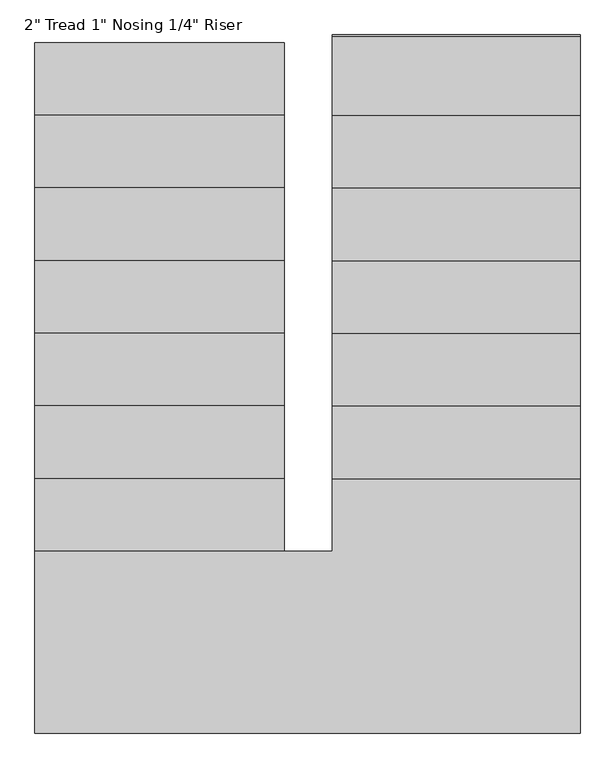
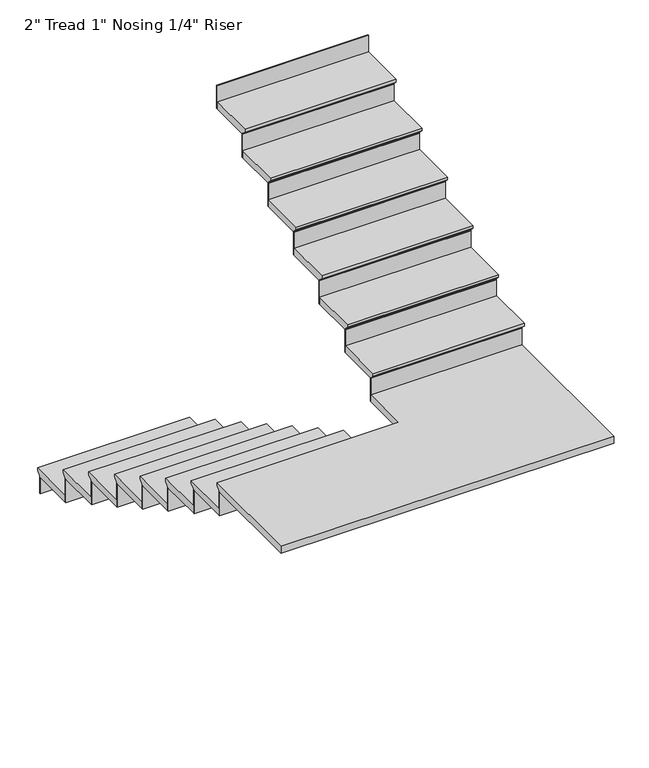
"""IFC4 building model written with IfcOpenShell, lengths in millimetres: stair flight geometry."""

from ifc_helpers import new_model, si_unit, origin, place, context, project, spatial, faceted_brep, source, transform, mapped, element, save


def stair_flight_c3010b6b(model_context):
    return source(origin(), model_context, "Body", "Brep", [
        faceted_brep([(-4232.280864, -3571.6080018, 6398.6833333), (-4232.280864, -3571.6080018, 6417.7333333), (-3187.6083919, -3571.6080018, 6417.7333333), (-3187.6083919, -3571.6080018, 6398.6833333), (-4232.280864, -3597.0080018, 6373.2833333), (-3187.6083919, -3597.0080018, 6373.2833333), (-4232.280864, -3901.8080018, 6417.7333333), (-3187.6083919, -3901.8080018, 6417.7333333), (-3187.6083919, -3597.0080018, 6366.9333333), (-3187.6083919, -3901.8080018, 6366.9333333), (-4232.280864, -3901.8080018, 6366.9333333), (-4232.280864, -3597.0080018, 6366.9333333)], [[[0, 1, 2, 3]], [[4, 0, 3, 5]], [[2, 1, 6, 7]], [[8, 9, 10, 11]], [[2, 7, 9, 8, 5, 3]], [[8, 11, 4, 5]], [[6, 1, 0, 4, 11, 10]], [[7, 6, 10, 9]]]),
        faceted_brep([(-4232.280864, -3597.0080018, 6366.9333333), (-4232.280864, -3597.0080018, 6248.4), (-4232.280864, -3603.3580018, 6248.4), (-4232.280864, -3603.3580018, 6366.9333333), (-3187.6083919, -3597.0080018, 6366.9333333), (-3187.6083919, -3603.3580018, 6366.9333333), (-3187.6083919, -3603.3580018, 6248.4), (-3187.6083919, -3597.0080018, 6248.4)], [[[0, 1, 2, 3]], [[4, 5, 6, 7]], [[1, 0, 4, 7]], [[2, 1, 7, 6]], [[3, 2, 6, 5]], [[0, 3, 5, 4]]]),
        faceted_brep([(-4232.280864, -3901.8080018, 6536.2666667), (-4232.280864, -3901.8080018, 6366.9333333), (-4232.280864, -3908.1580018, 6366.9333333), (-4232.280864, -3908.1580018, 6536.2666667), (-3187.6083919, -3901.8080018, 6536.2666667), (-3187.6083919, -3908.1580018, 6536.2666667), (-3187.6083919, -3908.1580018, 6366.9333333), (-3187.6083919, -3901.8080018, 6366.9333333)], [[[0, 1, 2, 3]], [[4, 5, 6, 7]], [[1, 0, 4, 7]], [[2, 1, 7, 6]], [[3, 2, 6, 5]], [[0, 3, 5, 4]]]),
        faceted_brep([(-3187.6083919, -3876.4080018, 6587.0666667), (-4232.280864, -3876.4080018, 6587.0666667), (-4232.280864, -4206.6080018, 6587.0666667), (-3187.6083919, -4206.6080018, 6587.0666667), (-3187.6083919, -3901.8080018, 6536.2666667), (-3187.6083919, -4206.6080018, 6536.2666667), (-4232.280864, -4206.6080018, 6536.2666667), (-4232.280864, -3901.8080018, 6536.2666667), (-3187.6083919, -3901.8080018, 6542.6166667), (-3187.6083919, -3876.4080018, 6568.0166667), (-4232.280864, -3901.8080018, 6542.6166667), (-4232.280864, -3876.4080018, 6568.0166667)], [[[0, 1, 2, 3]], [[4, 5, 6, 7]], [[0, 3, 5, 4, 8, 9]], [[4, 7, 10, 8]], [[2, 1, 11, 10, 7, 6]], [[3, 2, 6, 5]], [[11, 1, 0, 9]], [[10, 11, 9, 8]]]),
        faceted_brep([(-4232.280864, -4206.6080018, 6705.6), (-4232.280864, -4206.6080018, 6536.2666667), (-4232.280864, -4212.9580018, 6536.2666667), (-4232.280864, -4212.9580018, 6705.6), (-3187.6083919, -4206.6080018, 6705.6), (-3187.6083919, -4212.9580018, 6705.6), (-3187.6083919, -4212.9580018, 6536.2666667), (-3187.6083919, -4206.6080018, 6536.2666667)], [[[0, 1, 2, 3]], [[4, 5, 6, 7]], [[1, 0, 4, 7]], [[2, 1, 7, 6]], [[3, 2, 6, 5]], [[0, 3, 5, 4]]]),
        faceted_brep([(-3187.6083919, -4181.2080018, 6756.4), (-4232.280864, -4181.2080018, 6756.4), (-4232.280864, -4511.4080018, 6756.4), (-3187.6083919, -4511.4080018, 6756.4), (-3187.6083919, -4206.6080018, 6705.6), (-3187.6083919, -4511.4080018, 6705.6), (-4232.280864, -4511.4080018, 6705.6), (-4232.280864, -4206.6080018, 6705.6), (-3187.6083919, -4206.6080018, 6711.95), (-3187.6083919, -4181.2080018, 6737.35), (-4232.280864, -4206.6080018, 6711.95), (-4232.280864, -4181.2080018, 6737.35)], [[[0, 1, 2, 3]], [[4, 5, 6, 7]], [[0, 3, 5, 4, 8, 9]], [[4, 7, 10, 8]], [[2, 1, 11, 10, 7, 6]], [[3, 2, 6, 5]], [[11, 1, 0, 9]], [[10, 11, 9, 8]]]),
        faceted_brep([(-4232.280864, -4511.4080018, 6874.9333333), (-4232.280864, -4511.4080018, 6705.6), (-4232.280864, -4517.7580018, 6705.6), (-4232.280864, -4517.7580018, 6874.9333333), (-3187.6083919, -4511.4080018, 6874.9333333), (-3187.6083919, -4517.7580018, 6874.9333333), (-3187.6083919, -4517.7580018, 6705.6), (-3187.6083919, -4511.4080018, 6705.6)], [[[0, 1, 2, 3]], [[4, 5, 6, 7]], [[1, 0, 4, 7]], [[2, 1, 7, 6]], [[3, 2, 6, 5]], [[0, 3, 5, 4]]]),
        faceted_brep([(-3187.6083919, -4486.0080018, 6925.7333333), (-4232.280864, -4486.0080018, 6925.7333333), (-4232.280864, -4816.2080018, 6925.7333333), (-3187.6083919, -4816.2080018, 6925.7333333), (-3187.6083919, -4511.4080018, 6874.9333333), (-3187.6083919, -4816.2080018, 6874.9333333), (-4232.280864, -4816.2080018, 6874.9333333), (-4232.280864, -4511.4080018, 6874.9333333), (-3187.6083919, -4511.4080018, 6881.2833333), (-3187.6083919, -4486.0080018, 6906.6833333), (-4232.280864, -4511.4080018, 6881.2833333), (-4232.280864, -4486.0080018, 6906.6833333)], [[[0, 1, 2, 3]], [[4, 5, 6, 7]], [[0, 3, 5, 4, 8, 9]], [[4, 7, 10, 8]], [[2, 1, 11, 10, 7, 6]], [[3, 2, 6, 5]], [[11, 1, 0, 9]], [[10, 11, 9, 8]]]),
        faceted_brep([(-4232.280864, -4816.2080018, 7044.2666667), (-4232.280864, -4816.2080018, 6874.9333333), (-4232.280864, -4822.5580018, 6874.9333333), (-4232.280864, -4822.5580018, 7044.2666667), (-3187.6083919, -4816.2080018, 7044.2666667), (-3187.6083919, -4822.5580018, 7044.2666667), (-3187.6083919, -4822.5580018, 6874.9333333), (-3187.6083919, -4816.2080018, 6874.9333333)], [[[0, 1, 2, 3]], [[4, 5, 6, 7]], [[1, 0, 4, 7]], [[2, 1, 7, 6]], [[3, 2, 6, 5]], [[0, 3, 5, 4]]]),
        faceted_brep([(-3187.6083919, -4790.8080018, 7095.0666667), (-4232.280864, -4790.8080018, 7095.0666667), (-4232.280864, -5121.0080018, 7095.0666667), (-3187.6083919, -5121.0080018, 7095.0666667), (-3187.6083919, -4816.2080018, 7044.2666667), (-3187.6083919, -5121.0080018, 7044.2666667), (-4232.280864, -5121.0080018, 7044.2666667), (-4232.280864, -4816.2080018, 7044.2666667), (-3187.6083919, -4816.2080018, 7050.6166667), (-3187.6083919, -4790.8080018, 7076.0166667), (-4232.280864, -4816.2080018, 7050.6166667), (-4232.280864, -4790.8080018, 7076.0166667)], [[[0, 1, 2, 3]], [[4, 5, 6, 7]], [[0, 3, 5, 4, 8, 9]], [[4, 7, 10, 8]], [[2, 1, 11, 10, 7, 6]], [[3, 2, 6, 5]], [[11, 1, 0, 9]], [[10, 11, 9, 8]]]),
        faceted_brep([(-4232.280864, -5121.0080018, 7213.6), (-4232.280864, -5121.0080018, 7044.2666667), (-4232.280864, -5127.3580018, 7044.2666667), (-4232.280864, -5127.3580018, 7213.6), (-3187.6083919, -5121.0080018, 7213.6), (-3187.6083919, -5127.3580018, 7213.6), (-3187.6083919, -5127.3580018, 7044.2666667), (-3187.6083919, -5121.0080018, 7044.2666667)], [[[0, 1, 2, 3]], [[4, 5, 6, 7]], [[1, 0, 4, 7]], [[2, 1, 7, 6]], [[3, 2, 6, 5]], [[0, 3, 5, 4]]]),
        faceted_brep([(-3187.6083919, -5095.6080018, 7264.4), (-4232.280864, -5095.6080018, 7264.4), (-4232.280864, -5425.8080018, 7264.4), (-3187.6083919, -5425.8080018, 7264.4), (-3187.6083919, -5121.0080018, 7213.6), (-3187.6083919, -5425.8080018, 7213.6), (-4232.280864, -5425.8080018, 7213.6), (-4232.280864, -5121.0080018, 7213.6), (-3187.6083919, -5121.0080018, 7219.95), (-3187.6083919, -5095.6080018, 7245.35), (-4232.280864, -5121.0080018, 7219.95), (-4232.280864, -5095.6080018, 7245.35)], [[[0, 1, 2, 3]], [[4, 5, 6, 7]], [[0, 3, 5, 4, 8, 9]], [[4, 7, 10, 8]], [[2, 1, 11, 10, 7, 6]], [[3, 2, 6, 5]], [[11, 1, 0, 9]], [[10, 11, 9, 8]]]),
        faceted_brep([(-4232.280864, -5425.8080018, 7382.9333333), (-4232.280864, -5425.8080018, 7213.6), (-4232.280864, -5432.1580018, 7213.6), (-4232.280864, -5432.1580018, 7382.9333333), (-3187.6083919, -5425.8080018, 7382.9333333), (-3187.6083919, -5432.1580018, 7382.9333333), (-3187.6083919, -5432.1580018, 7213.6), (-3187.6083919, -5425.8080018, 7213.6)], [[[0, 1, 2, 3]], [[4, 5, 6, 7]], [[1, 0, 4, 7]], [[2, 1, 7, 6]], [[3, 2, 6, 5]], [[0, 3, 5, 4]]]),
        faceted_brep([(-3187.6083919, -5400.4080018, 7433.7333333), (-4232.280864, -5400.4080018, 7433.7333333), (-4232.280864, -5730.6080018, 7433.7333333), (-3187.6083919, -5730.6080018, 7433.7333333), (-3187.6083919, -5425.8080018, 7382.9333333), (-3187.6083919, -5730.6080018, 7382.9333333), (-4232.280864, -5730.6080018, 7382.9333333), (-4232.280864, -5425.8080018, 7382.9333333), (-3187.6083919, -5425.8080018, 7389.2833333), (-3187.6083919, -5400.4080018, 7414.6833333), (-4232.280864, -5425.8080018, 7389.2833333), (-4232.280864, -5400.4080018, 7414.6833333)], [[[0, 1, 2, 3]], [[4, 5, 6, 7]], [[0, 3, 5, 4, 8, 9]], [[4, 7, 10, 8]], [[2, 1, 11, 10, 7, 6]], [[3, 2, 6, 5]], [[11, 1, 0, 9]], [[10, 11, 9, 8]]]),
        faceted_brep([(-4232.280864, -5730.6080018, 7552.2666667), (-4232.280864, -5730.6080018, 7382.9333333), (-4232.280864, -5736.9580018, 7382.9333333), (-4232.280864, -5736.9580018, 7552.2666667), (-3187.6083919, -5730.6080018, 7552.2666667), (-3187.6083919, -5736.9580018, 7552.2666667), (-3187.6083919, -5736.9580018, 7382.9333333), (-3187.6083919, -5730.6080018, 7382.9333333)], [[[0, 1, 2, 3]], [[4, 5, 6, 7]], [[1, 0, 4, 7]], [[2, 1, 7, 6]], [[3, 2, 6, 5]], [[0, 3, 5, 4]]]),
        faceted_brep([(-2984.4083919, -5375.0080018, 7603.0666667), (-2984.4083919, -5705.2080018, 7603.0666667), (-4232.280864, -5705.2080018, 7603.0666667), (-4232.280864, -6467.2080018, 7603.0666667), (-1946.280864, -6467.2080018, 7603.0666667), (-1946.280864, -5375.0080018, 7603.0666667), (-2984.4083919, -5705.2080018, 7552.2666667), (-2984.4083919, -5375.0080018, 7552.2666667), (-1946.280864, -5375.0080018, 7552.2666667), (-1946.280864, -6467.2080018, 7552.2666667), (-4232.280864, -6467.2080018, 7552.2666667), (-4232.280864, -5730.6080018, 7552.2666667), (-3187.6083919, -5730.6080018, 7552.2666667), (-3187.6083919, -5705.2080018, 7552.2666667), (-3187.6083919, -5705.2080018, 7584.0166667), (-4232.280864, -5705.2080018, 7584.0166667), (-3187.6083919, -5730.6080018, 7558.6166667), (-4232.280864, -5730.6080018, 7558.6166667)], [[[0, 1, 2, 3, 4, 5]], [[6, 7, 8, 9, 10, 11, 12, 13]], [[1, 0, 7, 6]], [[2, 1, 6, 13, 14, 15]], [[13, 12, 16, 14]], [[12, 11, 17, 16]], [[3, 2, 15, 17, 11, 10]], [[4, 3, 10, 9]], [[5, 4, 9, 8]], [[0, 5, 8, 7]], [[17, 15, 14, 16]]]),
        faceted_brep([(-1946.280864, -5375.0080018, 7721.6), (-1946.280864, -5375.0080018, 7552.2666667), (-1946.280864, -5368.6580018, 7552.2666667), (-1946.280864, -5368.6580018, 7721.6), (-2984.4083919, -5375.0080018, 7721.6), (-2984.4083919, -5368.6580018, 7721.6), (-2984.4083919, -5368.6580018, 7552.2666667), (-2984.4083919, -5375.0080018, 7552.2666667)], [[[0, 1, 2, 3]], [[4, 5, 6, 7]], [[1, 0, 4, 7]], [[2, 1, 7, 6]], [[3, 2, 6, 5]], [[0, 3, 5, 4]]]),
        faceted_brep([(-2984.4083919, -5400.4080018, 7772.4), (-1946.280864, -5400.4080018, 7772.4), (-1946.280864, -5070.2080018, 7772.4), (-2984.4083919, -5070.2080018, 7772.4), (-2984.4083919, -5375.0080018, 7721.6), (-2984.4083919, -5070.2080018, 7721.6), (-1946.280864, -5070.2080018, 7721.6), (-1946.280864, -5375.0080018, 7721.6), (-2984.4083919, -5375.0080018, 7727.95), (-2984.4083919, -5400.4080018, 7753.35), (-1946.280864, -5375.0080018, 7727.95), (-1946.280864, -5400.4080018, 7753.35)], [[[0, 1, 2, 3]], [[4, 5, 6, 7]], [[0, 3, 5, 4, 8, 9]], [[4, 7, 10, 8]], [[2, 1, 11, 10, 7, 6]], [[3, 2, 6, 5]], [[11, 1, 0, 9]], [[10, 11, 9, 8]]]),
        faceted_brep([(-1946.280864, -5070.2080018, 7890.9333333), (-1946.280864, -5070.2080018, 7721.6), (-1946.280864, -5063.8580018, 7721.6), (-1946.280864, -5063.8580018, 7890.9333333), (-2984.4083919, -5070.2080018, 7890.9333333), (-2984.4083919, -5063.8580018, 7890.9333333), (-2984.4083919, -5063.8580018, 7721.6), (-2984.4083919, -5070.2080018, 7721.6)], [[[0, 1, 2, 3]], [[4, 5, 6, 7]], [[1, 0, 4, 7]], [[2, 1, 7, 6]], [[3, 2, 6, 5]], [[0, 3, 5, 4]]]),
        faceted_brep([(-2984.4083919, -5095.6080018, 7941.7333333), (-1946.280864, -5095.6080018, 7941.7333333), (-1946.280864, -4765.4080018, 7941.7333333), (-2984.4083919, -4765.4080018, 7941.7333333), (-2984.4083919, -5070.2080018, 7890.9333333), (-2984.4083919, -4765.4080018, 7890.9333333), (-1946.280864, -4765.4080018, 7890.9333333), (-1946.280864, -5070.2080018, 7890.9333333), (-2984.4083919, -5070.2080018, 7897.2833333), (-2984.4083919, -5095.6080018, 7922.6833333), (-1946.280864, -5070.2080018, 7897.2833333), (-1946.280864, -5095.6080018, 7922.6833333)], [[[0, 1, 2, 3]], [[4, 5, 6, 7]], [[0, 3, 5, 4, 8, 9]], [[4, 7, 10, 8]], [[2, 1, 11, 10, 7, 6]], [[3, 2, 6, 5]], [[11, 1, 0, 9]], [[10, 11, 9, 8]]]),
        faceted_brep([(-1946.280864, -4765.4080018, 8060.2666667), (-1946.280864, -4765.4080018, 7890.9333333), (-1946.280864, -4759.0580018, 7890.9333333), (-1946.280864, -4759.0580018, 8060.2666667), (-2984.4083919, -4765.4080018, 8060.2666667), (-2984.4083919, -4759.0580018, 8060.2666667), (-2984.4083919, -4759.0580018, 7890.9333333), (-2984.4083919, -4765.4080018, 7890.9333333)], [[[0, 1, 2, 3]], [[4, 5, 6, 7]], [[1, 0, 4, 7]], [[2, 1, 7, 6]], [[3, 2, 6, 5]], [[0, 3, 5, 4]]]),
        faceted_brep([(-2984.4083919, -4790.8080018, 8111.0666667), (-1946.280864, -4790.8080018, 8111.0666667), (-1946.280864, -4460.6080018, 8111.0666667), (-2984.4083919, -4460.6080018, 8111.0666667), (-2984.4083919, -4765.4080018, 8060.2666667), (-2984.4083919, -4460.6080018, 8060.2666667), (-1946.280864, -4460.6080018, 8060.2666667), (-1946.280864, -4765.4080018, 8060.2666667), (-2984.4083919, -4765.4080018, 8066.6166667), (-2984.4083919, -4790.8080018, 8092.0166667), (-1946.280864, -4765.4080018, 8066.6166667), (-1946.280864, -4790.8080018, 8092.0166667)], [[[0, 1, 2, 3]], [[4, 5, 6, 7]], [[0, 3, 5, 4, 8, 9]], [[4, 7, 10, 8]], [[2, 1, 11, 10, 7, 6]], [[3, 2, 6, 5]], [[11, 1, 0, 9]], [[10, 11, 9, 8]]]),
        faceted_brep([(-1946.280864, -4460.6080018, 8229.6), (-1946.280864, -4460.6080018, 8060.2666667), (-1946.280864, -4454.2580018, 8060.2666667), (-1946.280864, -4454.2580018, 8229.6), (-2984.4083919, -4460.6080018, 8229.6), (-2984.4083919, -4454.2580018, 8229.6), (-2984.4083919, -4454.2580018, 8060.2666667), (-2984.4083919, -4460.6080018, 8060.2666667)], [[[0, 1, 2, 3]], [[4, 5, 6, 7]], [[1, 0, 4, 7]], [[2, 1, 7, 6]], [[3, 2, 6, 5]], [[0, 3, 5, 4]]]),
        faceted_brep([(-2984.4083919, -4486.0080018, 8280.4), (-1946.280864, -4486.0080018, 8280.4), (-1946.280864, -4155.8080018, 8280.4), (-2984.4083919, -4155.8080018, 8280.4), (-2984.4083919, -4460.6080018, 8229.6), (-2984.4083919, -4155.8080018, 8229.6), (-1946.280864, -4155.8080018, 8229.6), (-1946.280864, -4460.6080018, 8229.6), (-2984.4083919, -4460.6080018, 8235.95), (-2984.4083919, -4486.0080018, 8261.35), (-1946.280864, -4460.6080018, 8235.95), (-1946.280864, -4486.0080018, 8261.35)], [[[0, 1, 2, 3]], [[4, 5, 6, 7]], [[0, 3, 5, 4, 8, 9]], [[4, 7, 10, 8]], [[2, 1, 11, 10, 7, 6]], [[3, 2, 6, 5]], [[11, 1, 0, 9]], [[10, 11, 9, 8]]]),
        faceted_brep([(-1946.280864, -4155.8080018, 8398.9333333), (-1946.280864, -4155.8080018, 8229.6), (-1946.280864, -4149.4580018, 8229.6), (-1946.280864, -4149.4580018, 8398.9333333), (-2984.4083919, -4155.8080018, 8398.9333333), (-2984.4083919, -4149.4580018, 8398.9333333), (-2984.4083919, -4149.4580018, 8229.6), (-2984.4083919, -4155.8080018, 8229.6)], [[[0, 1, 2, 3]], [[4, 5, 6, 7]], [[1, 0, 4, 7]], [[2, 1, 7, 6]], [[3, 2, 6, 5]], [[0, 3, 5, 4]]]),
        faceted_brep([(-2984.4083919, -4181.2080018, 8449.7333333), (-1946.280864, -4181.2080018, 8449.7333333), (-1946.280864, -3851.0080018, 8449.7333333), (-2984.4083919, -3851.0080018, 8449.7333333), (-2984.4083919, -4155.8080018, 8398.9333333), (-2984.4083919, -3851.0080018, 8398.9333333), (-1946.280864, -3851.0080018, 8398.9333333), (-1946.280864, -4155.8080018, 8398.9333333), (-2984.4083919, -4155.8080018, 8405.2833333), (-2984.4083919, -4181.2080018, 8430.6833333), (-1946.280864, -4155.8080018, 8405.2833333), (-1946.280864, -4181.2080018, 8430.6833333)], [[[0, 1, 2, 3]], [[4, 5, 6, 7]], [[0, 3, 5, 4, 8, 9]], [[4, 7, 10, 8]], [[2, 1, 11, 10, 7, 6]], [[3, 2, 6, 5]], [[11, 1, 0, 9]], [[10, 11, 9, 8]]]),
        faceted_brep([(-1946.280864, -3851.0080018, 8568.2666667), (-1946.280864, -3851.0080018, 8398.9333333), (-1946.280864, -3844.6580018, 8398.9333333), (-1946.280864, -3844.6580018, 8568.2666667), (-2984.4083919, -3851.0080018, 8568.2666667), (-2984.4083919, -3844.6580018, 8568.2666667), (-2984.4083919, -3844.6580018, 8398.9333333), (-2984.4083919, -3851.0080018, 8398.9333333)], [[[0, 1, 2, 3]], [[4, 5, 6, 7]], [[1, 0, 4, 7]], [[2, 1, 7, 6]], [[3, 2, 6, 5]], [[0, 3, 5, 4]]]),
        faceted_brep([(-1946.280864, -3546.2080018, 8737.6), (-1946.280864, -3546.2080018, 8568.2666667), (-1946.280864, -3539.8580018, 8568.2666667), (-1946.280864, -3539.8580018, 8737.6), (-2984.4083919, -3546.2080018, 8737.6), (-2984.4083919, -3539.8580018, 8737.6), (-2984.4083919, -3539.8580018, 8568.2666667), (-2984.4083919, -3546.2080018, 8568.2666667)], [[[0, 1, 2, 3]], [[4, 5, 6, 7]], [[1, 0, 4, 7]], [[2, 1, 7, 6]], [[3, 2, 6, 5]], [[0, 3, 5, 4]]]),
        faceted_brep([(-2984.4083919, -3876.4080018, 8619.0666667), (-1946.280864, -3876.4080018, 8619.0666667), (-1946.280864, -3546.2080018, 8619.0666667), (-2984.4083919, -3546.2080018, 8619.0666667), (-2984.4083919, -3851.0080018, 8568.2666667), (-2984.4083919, -3546.2080018, 8568.2666667), (-1946.280864, -3546.2080018, 8568.2666667), (-1946.280864, -3851.0080018, 8568.2666667), (-2984.4083919, -3851.0080018, 8574.6166667), (-2984.4083919, -3876.4080018, 8600.0166667), (-1946.280864, -3851.0080018, 8574.6166667), (-1946.280864, -3876.4080018, 8600.0166667)], [[[0, 1, 2, 3]], [[4, 5, 6, 7]], [[0, 3, 5, 4, 8, 9]], [[4, 7, 10, 8]], [[2, 1, 11, 10, 7, 6]], [[3, 2, 6, 5]], [[11, 1, 0, 9]], [[10, 11, 9, 8]]]),
    ])


if __name__ == "__main__":
    model = new_model("IFC4")
    model_context = context("Model", 3, world=origin())
    ifc_project = project(units=[si_unit("LENGTHUNIT", "METRE", prefix="MILLI")], contexts=[model_context])
    site = spatial("IfcSite", under=ifc_project)
    building = spatial("IfcBuilding", under=site)
    placement = place(None, origin())
    stair_flight_shape = stair_flight_c3010b6b(model_context)
    element("IfcStairFlight", 1, ObjectType="2\" Tread 1\" Nosing 1/4\" Riser", at=placement, inside=building, context=model_context, shape_type="MappedRepresentation", body=[
        mapped(stair_flight_shape, transform((0.0, 0.0, 0.0), x_axis=(1.0, 0.0, 0.0), y_axis=(0.0, 1.0, 0.0), z_axis=(0.0, 0.0, 1.0))),
    ])
    save(model, "model.ifc")
